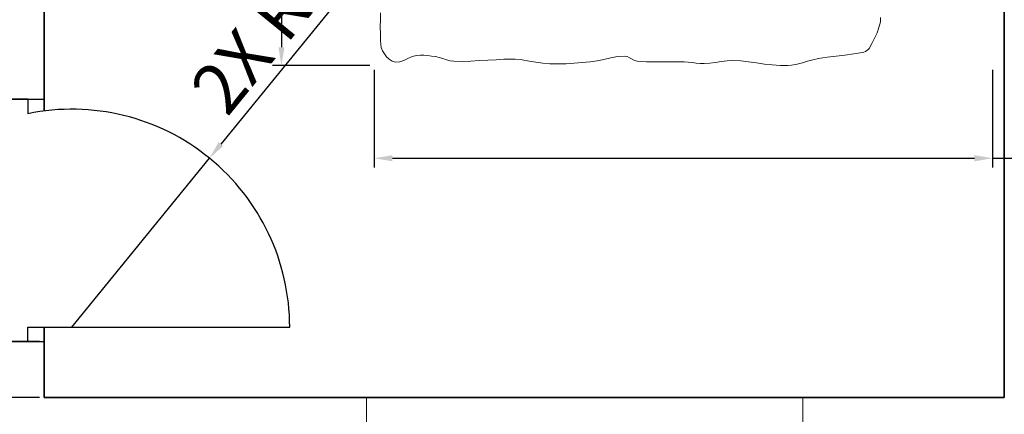
# Model space of a CAD drawing. Units: inches. Extents: x 1484 to 2008, y 1843 to 2590.
# Tile 3 of 21: x 1756 to 1891, y 1926 to 1981. Entities that reach past the tile are written whole.
import ezdxf

# ---------------------------------------------------------------- set-up
doc = ezdxf.new("R2010")
doc.units = ezdxf.units.IN
for name, color, linetype, lineweight in [('A-ANNO-DIMS', 2, 'Continuous', 18), ('A-DOOR', 4, 'Continuous', 25), ('A-FURN', 8, 'Continuous', 18), ('A-GLAZ', 4, 'Continuous', 18), ('A-WALL', 7, 'Continuous', 35)]:
    doc.layers.add(name, color=color, linetype=linetype, lineweight=lineweight)
doc.styles.get("Standard").update_dxf_attribs({"font": 'arial.ttf'})
doc.dimstyles.new('ISO-25', dxfattribs={"dimtxt": 7, "dimasz": 2.5, "dimexe": 1.25, "dimexo": 0.625, "dimtad": 1, "dimdec": 0, "dimlunit": 3, "dimtxsty": 'Standard', "dimcen": 2.5, "dimadec": 0, "dimazin": 0, "dimtfac": 1, "dimtdec": 0, "dimtmove": 0, "dimatfit": 3, "dimfxl": 1, "dimarcsym": 0})

# ---------------------------------------------------------------- blocks, each defined once
blk = doc.blocks.new('BED-DOUBLE')
for p, q in [((53.89, 69.59), (53.3, 69.63)), ((54.66, 69.4), (53.89, 69.59)), ((55.42, 69.13), (54.66, 69.4)), ((56.15, 68.8), (55.42, 69.13)), ((56.86, 68.43), (56.15, 68.8)), ((57.56, 68.03), (56.86, 68.43)), ((57.72, 67.9), (57.56, 68.03)), ((57.86, 67.73), (57.72, 67.9)), ((57.97, 67.54), (57.86, 67.73)), ((58.05, 67.33), (57.97, 67.54)), ((58.11, 67.12), (58.05, 67.33)), ((58.31, 65.92), (58.11, 67.12)), ((58.48, 64.7), (58.31, 65.92)), ((58.62, 63.49), (58.48, 64.7)), ((58.77, 62.27), (58.62, 63.49)), ((58.96, 61.06), (58.77, 62.27)), ((59.12, 60.32), (58.96, 61.06)), ((59.32, 59.59), (59.12, 60.32)), ((59.52, 58.87), (59.32, 59.59)), ((59.71, 58.13), (59.52, 58.87)), ((59.84, 57.39), (59.71, 58.13)), ((59.89, 56.86), (59.84, 57.39)), ((59.9, 56.33), (59.89, 56.86)), ((59.85, 55.26), (59.88, 55.79)), ((59.88, 55.79), (59.9, 56.33)), ((59.7, 53.64), (59.81, 54.72)), ((59.81, 54.72), (59.85, 55.26)), ((59.55, 52.56), (59.7, 53.64)), ((59.28, 50.39), (59.4, 51.47)), ((59.4, 51.47), (59.55, 52.56)), ((59.21, 49.3), (59.28, 50.39)), ((59.25, 48.51), (59.21, 49.3)), ((59.34, 47.72), (59.25, 48.51)), ((59.47, 46.94), (59.34, 47.72)), ((59.58, 46.15), (59.47, 46.94)), ((59.64, 45.36), (59.58, 46.15)), ((59.58, 44.26), (59.63, 44.81)), ((59.63, 44.81), (59.64, 45.36)), ((59.45, 43.17), (59.51, 43.71)), ((59.51, 43.71), (59.58, 44.26)), ((59.39, 41.32), (59.41, 42.62)), ((59.41, 42.62), (59.45, 43.17)), ((59.4, 40.03), (59.39, 41.32)), ((59.41, 38.74), (59.4, 40.03)), ((59.39, 37.44), (59.41, 38.74)), ((59.3, 36.15), (59.39, 37.44)), ((58.83, 35.11), (59.03, 35.45)), ((59.03, 35.45), (59.21, 35.79)), ((59.21, 35.79), (59.3, 36.15)), ((58.61, 34.41), (58.67, 34.77)), ((58.68, 33.46), (58.61, 34.41)), ((58.67, 34.77), (58.83, 35.11)), ((58.85, 32.52), (58.68, 33.46)), ((59.07, 31.59), (58.85, 32.52)), ((59.27, 30.66), (59.07, 31.59)), ((59.41, 29.71), (59.27, 30.66)), ((59.51, 28.6), (59.41, 29.71)), ((59.59, 27.49), (59.51, 28.6)), ((59.65, 26.38), (59.59, 27.49)), ((59.67, 25.26), (59.65, 26.38)), ((59.65, 24.15), (59.67, 25.26)), ((59.44, 22.24), (59.57, 23.19)), ((59.57, 23.19), (59.65, 24.15)), ((59.29, 21.29), (59.44, 22.24)), ((59.04, 19.39), (59.14, 20.34)), ((59.14, 20.34), (59.29, 21.29)), ((59.02, 18.86), (59.04, 19.39)), ((59.02, 18.34), (59.02, 18.86)), ((59.05, 17.81), (59.02, 18.34)), ((59.08, 17.28), (59.05, 17.81)), ((59.1, 16.75), (59.08, 17.28)), ((59.16, 15.6), (59.1, 16.75)), ((59.23, 14.44), (59.16, 15.6)), ((59.3, 13.28), (59.23, 14.44)), ((59.33, 12.12), (59.3, 13.28)), ((59.24, 10.44), (59.31, 10.96)), ((59.31, 10.96), (59.33, 12.12)), ((58.94, 9.43), (59.11, 9.93)), ((59.11, 9.93), (59.24, 10.44)), ((58.6, 7.89), (58.68, 8.41)), ((58.68, 8.41), (58.79, 8.92)), ((58.79, 8.92), (58.94, 9.43)), ((58.47, 6.32), (58.48, 6.84)), ((58.48, 6.84), (58.53, 7.36)), ((58.53, 7.36), (58.6, 7.89)), ((58.51, 5.8), (58.47, 6.32)), ((58.67, 5.21), (58.51, 5.8)), ((58.94, 4.64), (58.67, 5.21)), ((59.21, 4.08), (58.94, 4.64)), ((59.41, 3.51), (59.21, 4.08)), ((59.3, 2.47), (59.44, 2.92)), ((59.44, 2.92), (59.41, 3.51)), ((57.87, 1.14), (58.29, 1.39)), ((58.29, 1.39), (58.69, 1.7)), ((58.69, 1.7), (59.04, 2.06)), ((59.04, 2.06), (59.3, 2.47)), ((52.68, 0.86), (53.63, 0.84)), ((53.63, 0.84), (54.58, 0.83)), ((54.58, 0.83), (55.53, 0.85)), ((55.53, 0.85), (56.01, 0.86)), ((56.01, 0.86), (56.49, 0.86)), ((56.49, 0.86), (56.97, 0.89)), ((56.97, 0.89), (57.43, 0.97)), ((57.43, 0.97), (57.87, 1.14))]:
    blk.add_line(p, q)
blk = doc.blocks.new('DOOR-SWING-36IN')
for p, q in [((-2.25, 31.33), (2.25, 31.33)), ((0, 31.33), (0, 29.33)), ((0, -2), (0, 0)), ((0, 0), (36, 0)), ((-2.25, -2), (2.25, -2))]:
    blk.add_line(p, q)
blk.add_arc((6.05, 0), 29.95, 0, 101.6643)
blk = doc.blocks.new('WIN-60IN')
for p, q in [((0, 4.5), (0, -4.5)), ((60, 0), (60, 4.5)), ((60, 4.5), (60, -4.5)), ((0, -4.5), (0, 0)), ((0, 0), (60, 0))]:
    blk.add_line(p, q)
blk = doc.blocks.new('*D9')
at = {"layer": 'A-ANNO-DIMS', "color": 0, "lineweight": -2, "transparency": 16777216}
for p, q in [((1804.29, 1973.81), (1804.29, 1960.43)), ((1889.31, 1973.81), (1889.31, 1960.43)), ((1806.79, 1961.68), (1886.81, 1961.68)), ((1889.31, 1961.68), (2001.13, 1961.68))]:
    blk.add_line(p, q, dxfattribs=at)
at = {"layer": 'A-ANNO-DIMS', "color": 0, "transparency": 16777216}
for points in [[(1806.79, 1962.1), (1806.79, 1961.26), (1804.29, 1961.68)], [(1886.81, 1962.1), (1886.81, 1961.26), (1889.31, 1961.68)]]:
    blk.add_solid(points, dxfattribs=at)
at = {"layer": 'Defpoints', "color": 0, "transparency": 16777216}
for p in [(1804.29, 1974.43), (1889.31, 1974.43), (1889.31, 1961.68)]:
    blk.add_point(p, dxfattribs=at)
at = {"layer": 'A-ANNO-DIMS', "color": 0, "transparency": 16777216, "insert": (1946.47, 1965.93), "char_height": 7, "attachment_point": 5}
blk.add_mtext('DOUBLE BED 7\'-1" TYP.', dxfattribs=at)
blk = doc.blocks.new('*D10')
at = {"layer": 'A-ANNO-DIMS', "color": 0, "lineweight": -2, "transparency": 16777216}
for p, q in [((1803.67, 2034.33), (1790.29, 2034.33)), ((1791.54, 2031.83), (1791.54, 1976.93)), ((1803.67, 1974.43), (1790.29, 1974.43))]:
    blk.add_line(p, q, dxfattribs=at)
at = {"layer": 'A-ANNO-DIMS', "color": 0, "transparency": 16777216}
for points in [[(1791.12, 2031.83), (1791.95, 2031.83), (1791.54, 2034.33)], [(1791.12, 1976.93), (1791.95, 1976.93), (1791.54, 1974.43)]]:
    blk.add_solid(points, dxfattribs=at)
at = {"layer": 'Defpoints', "color": 0, "transparency": 16777216}
for p in [(1804.29, 2034.33), (1791.54, 1974.43), (1804.29, 1974.43)]:
    blk.add_point(p, dxfattribs=at)
at = {"layer": 'A-ANNO-DIMS', "color": 0, "transparency": 16777216, "insert": (1787.34, 2004.38), "char_height": 7, "attachment_point": 5, "rotation": 90}
blk.add_mtext('5\'-0" TYP.', dxfattribs=at)
blk = doc.blocks.new('*D40')
at = {"layer": 'A-ANNO-DIMS', "color": 0, "lineweight": -2, "transparency": 16777216}
for p, q in [((1739.37, 1936.47), (1739.37, 1975.14)), ((1758.29, 1936.47), (1738.12, 1936.47)), ((1739.37, 1931.3), (1739.37, 1933.97)), ((1758.29, 1928.8), (1738.12, 1928.8))]:
    blk.add_line(p, q, dxfattribs=at)
at = {"layer": 'A-ANNO-DIMS', "color": 0, "transparency": 16777216}
for points in [[(1738.95, 1933.97), (1739.79, 1933.97), (1739.37, 1936.47)], [(1738.95, 1931.3), (1739.79, 1931.3), (1739.37, 1928.8)]]:
    blk.add_solid(points, dxfattribs=at)
at = {"layer": 'Defpoints', "color": 0, "transparency": 16777216}
for p in [(1739.37, 1936.47), (1758.92, 1936.47), (1758.92, 1928.8)]:
    blk.add_point(p, dxfattribs=at)
at = {"layer": 'A-ANNO-DIMS', "color": 0, "transparency": 16777216, "insert": (1735.13, 1957.05), "char_height": 7, "attachment_point": 5, "rotation": 90}
blk.add_mtext('0\'-7 1/2"', dxfattribs=at)
blk = doc.blocks.new('*D65')
at = {"layer": 'A-ANNO-DIMS', "color": 0, "lineweight": -2, "transparency": 16777216}
for p, q in [((1811.14, 1997.91), (1783.22, 1963.63)), ((1762.72, 1938.47), (1781.64, 1961.69))]:
    blk.add_line(p, q, dxfattribs=at)
at = {"layer": 'A-ANNO-DIMS', "color": 0, "transparency": 16777216}
blk.add_solid([(1782.89, 1963.89), (1783.54, 1963.36), (1781.64, 1961.69)], dxfattribs=at)
at = {"layer": 'Defpoints', "color": 0, "transparency": 16777216}
for p in [(1781.64, 1961.69), (1762.72, 1938.47)]:
    blk.add_point(p, dxfattribs=at)
at = {"layer": 'A-ANNO-DIMS', "color": 0, "transparency": 16777216, "insert": (1794.71, 1984.39), "char_height": 7, "attachment_point": 5, "rotation": 50.833}
blk.add_mtext('2X R2\'-6"', dxfattribs=at)

msp = doc.modelspace()

# ---------------------------------------------------------------- linework, layer by layer
at = {"layer": 'A-DOOR'}
msp.add_line((1756.67, 1969.8), (1754.42, 1969.8), dxfattribs=at)
at = {"layer": 'A-WALL'}
for p, q in [((1758.92, 2072.8), (1758.92, 1968.17)), ((1890.92, 2072.8), (1890.92, 1928.8)), ((1758.92, 2060.81), (1758.92, 1968.17)), ((1758.92, 1938.47), (1758.92, 1929.81)), ((1758.92, 1938.47), (1758.92, 1928.8)), ((1758.92, 1928.8), (1890.92, 1928.8))]:
    msp.add_line(p, q, dxfattribs=at)

# ---------------------------------------------------------------- block references
at = {"layer": 'A-DOOR'}
msp.add_blockref('DOOR-SWING-36IN', (1756.67, 1938.47), dxfattribs=at)
at = {"layer": 'A-FURN', "rotation": 269.9999999999906}
msp.add_blockref('BED-DOUBLE', (1804.29, 2034.33), dxfattribs=at)
at = {"layer": 'A-GLAZ', "rotation": 180}
msp.add_blockref('WIN-60IN', (1863.22, 1924.3), dxfattribs=at)

# ---------------------------------------------------------------- dimensions: what is measured, and where the dimension line sits
at = {"layer": 'A-ANNO-DIMS'}
dim = msp.add_linear_dim(base=(1791.54, 1974.43), p1=(1804.29, 2034.33), p2=(1804.29, 1974.43), angle=270, text='<> TYP.', dimstyle='ISO-25', override={"dimdec": 1, "dimlfac": 1, "dimrnd": 0, "dimzin": 1, "dimdsep": 46, "dimlunit": 4, "dimfrac": 2}, dxfattribs=at)
dim.commit()
dim.dimension.update_dxf_attribs({"geometry": '*D10', "text_midpoint": (1787.34, 2004.38)})
dim = msp.add_radius_dim(center=(1762.724, 1938.47), mpoint=(1781.6371, 1961.6872), text='2X <>', dimstyle='ISO-25', override={"dimdec": 1, "dimlfac": 1, "dimrnd": 0, "dimzin": 1, "dimdsep": 46, "dimlunit": 4, "dimfrac": 2}, dxfattribs=at)
dim.commit()
dim.dimension.update_dxf_attribs({"geometry": '*D65', "text_midpoint": (1794.7135, 1984.3876)})
dim = msp.add_linear_dim(base=(1889.31, 1961.68), p1=(1804.29, 1974.43), p2=(1889.31, 1974.43), text='DOUBLE BED <> TYP.', dimstyle='ISO-25', override={"dimdec": 1, "dimlfac": 1, "dimrnd": 0, "dimzin": 1, "dimdsep": 46, "dimlunit": 4, "dimfrac": 2}, dxfattribs=at)
dim.commit()
dim.dimension.update_dxf_attribs({"geometry": '*D9', "text_midpoint": (1946.47, 1965.93)})
dim = msp.add_linear_dim(base=(1739.37, 1936.47), p1=(1758.92, 1928.8), p2=(1758.92, 1936.47), angle=90, dimstyle='ISO-25', override={"dimdec": 1, "dimlfac": 1, "dimrnd": 0, "dimzin": 1, "dimdsep": 46, "dimlunit": 4, "dimfrac": 2}, dxfattribs=at)
dim.commit()
dim.dimension.update_dxf_attribs({"geometry": '*D40', "text_midpoint": (1735.13, 1957.05)})

doc.saveas('drawing.dxf')
